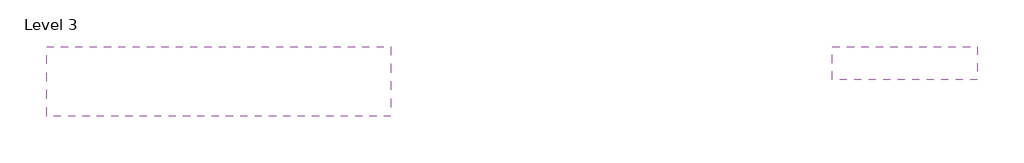
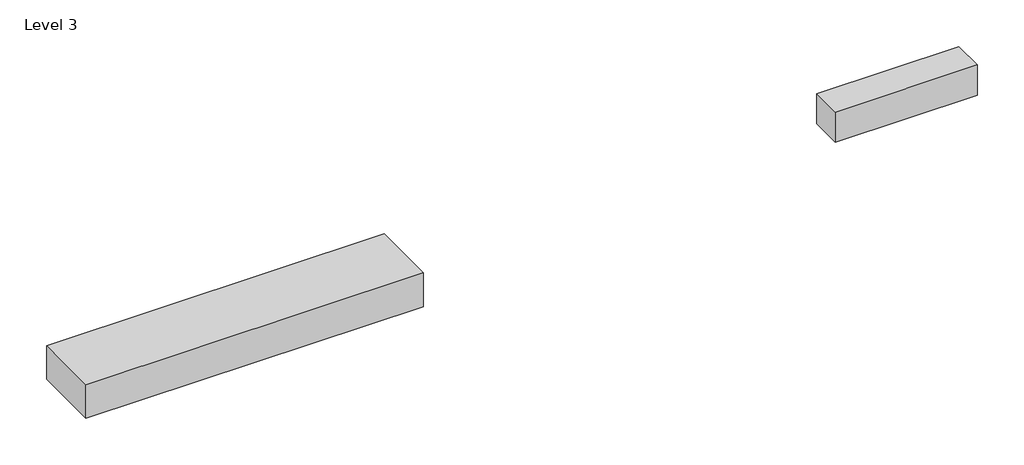
# One storey: 2 proxies.
"""IFC4 building model written with IfcOpenShell, lengths in millimetres."""

from ifc_helpers import new_model, si_unit, origin, place, context, project, spatial, transform, mapped, element, save
from components import generic_models_5_generic_models_5_ea9a58cb, generic_models_6_generic_models_6_f1c04d34

model = new_model("IFC4")

# Units and contexts
model_context = context("Model", 3, world=origin())
ifc_project = project(units=[si_unit("LENGTHUNIT", "METRE", prefix="MILLI")], contexts=[model_context])

# Site, building, storey
site = spatial("IfcSite", under=ifc_project)
building = spatial("IfcBuilding", under=site)
storey = spatial("IfcBuildingStorey", under=building, Name="Level 3", Elevation=3276.6)

# Proxies
placement = place(None, origin())
generic_models_5_generic_models_5_shape = generic_models_5_generic_models_5_ea9a58cb(model_context)
element("IfcBuildingElementProxy", 1, Name="Generic Models 5 : Generic Models 5", ObjectType="Generic Models 5 : Generic Models 5", at=placement, inside=storey, context=model_context, shape_type="MappedRepresentation", body=[
    mapped(generic_models_5_generic_models_5_shape, transform((0.0, 0.0, 0.0), x_axis=(1.0, 0.0, 0.0), y_axis=(0.0, 1.0, 0.0), z_axis=(0.0, 0.0, 1.0))),
])
generic_models_6_generic_models_6_shape = generic_models_6_generic_models_6_f1c04d34(model_context)
element("IfcBuildingElementProxy", 2, Name="Generic Models 6 : Generic Models 6", ObjectType="Generic Models 6 : Generic Models 6", at=placement, inside=storey, context=model_context, shape_type="MappedRepresentation", body=[
    mapped(generic_models_6_generic_models_6_shape, transform((0.0, 0.0, 0.0), x_axis=(1.0, 0.0, 0.0), y_axis=(0.0, 1.0, 0.0), z_axis=(0.0, 0.0, 1.0))),
])

save(model, "model.ifc")

# Revit data of these elements
# Element 1 (IfcBuildingElementProxy, "Generic Models 5 : Generic Models 5")
#   Phase Created = New Construction
# Element 2 (IfcBuildingElementProxy, "Generic Models 6 : Generic Models 6")
#   Phase Created = New Construction
